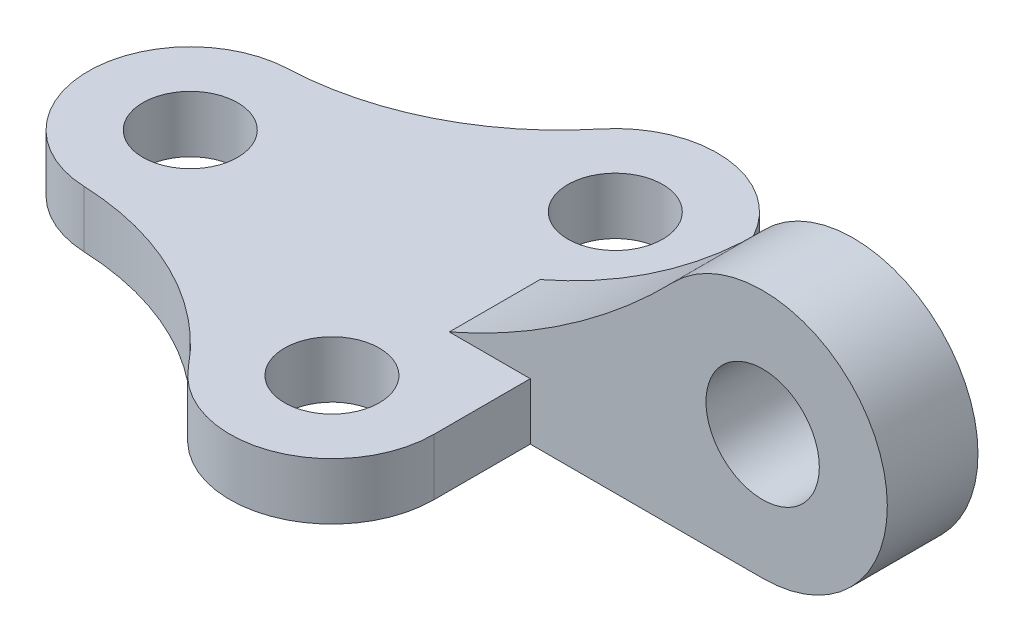
ISO-10303-21;
HEADER;
FILE_DESCRIPTION(('STEP AP214'),'2;1');
FILE_NAME('part.step','',(''),(''),'','','');
FILE_SCHEMA(('AUTOMOTIVE_DESIGN { 1 0 10303 214 1 1 1 1 }'));
ENDSEC;
DATA;
#1=APPLICATION_CONTEXT('core data for automotive mechanical design processes');
#2=APPLICATION_PROTOCOL_DEFINITION('international standard','automotive_design',2000,#1);
#3=PRODUCT_CONTEXT('',#1,'mechanical');
#4=PRODUCT('Part','Part','',(#3));
#5=PRODUCT_RELATED_PRODUCT_CATEGORY('part','',(#4));
#6=PRODUCT_DEFINITION_FORMATION('','',#4);
#7=PRODUCT_DEFINITION_CONTEXT('part definition',#1,'design');
#8=PRODUCT_DEFINITION('design','',#6,#7);
#9=PRODUCT_DEFINITION_SHAPE('','',#8);
#10=(LENGTH_UNIT() NAMED_UNIT(*) SI_UNIT(.MILLI.,.METRE.));
#11=(NAMED_UNIT(*) PLANE_ANGLE_UNIT() SI_UNIT($,.RADIAN.));
#12=(NAMED_UNIT(*) SI_UNIT($,.STERADIAN.) SOLID_ANGLE_UNIT());
#13=UNCERTAINTY_MEASURE_WITH_UNIT(LENGTH_MEASURE(1.E-05),#10,'distance_accuracy_value','');
#14=(GEOMETRIC_REPRESENTATION_CONTEXT(3) GLOBAL_UNCERTAINTY_ASSIGNED_CONTEXT((#13)) GLOBAL_UNIT_ASSIGNED_CONTEXT((#10,
#11,#12)) REPRESENTATION_CONTEXT('',''));
#15=CARTESIAN_POINT('',(0.,0.,0.));
#16=DIRECTION('',(0.,0.,1.));
#17=DIRECTION('',(1.,0.,0.));
#18=AXIS2_PLACEMENT_3D('',#15,#16,#17);
#19=CARTESIAN_POINT('',(68.,10.,-25.));
#20=DIRECTION('',(-1.,0.,0.));
#21=DIRECTION('',(0.,0.,1.));
#22=AXIS2_PLACEMENT_3D('',#19,#20,#21);
#23=PLANE('',#22);
#24=DIRECTION('',(0.,-1.,0.));
#25=VECTOR('',#24,1.);
#26=CARTESIAN_POINT('',(68.,10.,-8.));
#27=LINE('',#26,#25);
#28=CARTESIAN_POINT('',(68.,10.,-8.));
#29=VERTEX_POINT('',#28);
#30=CARTESIAN_POINT('',(68.,0.,-8.));
#31=VERTEX_POINT('',#30);
#32=EDGE_CURVE('E152',#29,#31,#27,.T.);
#33=ORIENTED_EDGE('',*,*,#32,.T.);
#34=DIRECTION('',(0.,0.,-1.));
#35=VECTOR('',#34,1.);
#36=CARTESIAN_POINT('',(68.,0.,-25.));
#37=LINE('',#36,#35);
#38=CARTESIAN_POINT('',(68.,0.,-25.));
#39=VERTEX_POINT('',#38);
#40=EDGE_CURVE('E207',#31,#39,#37,.T.);
#41=ORIENTED_EDGE('',*,*,#40,.T.);
#42=DIRECTION('',(0.,-1.,0.));
#43=VECTOR('',#42,1.);
#44=CARTESIAN_POINT('',(68.,10.,-25.));
#45=LINE('',#44,#43);
#46=CARTESIAN_POINT('',(68.,10.,-25.));
#47=VERTEX_POINT('',#46);
#48=EDGE_CURVE('E214',#47,#39,#45,.T.);
#49=ORIENTED_EDGE('',*,*,#48,.F.);
#50=DIRECTION('',(0.,0.,-1.));
#51=VECTOR('',#50,1.);
#52=CARTESIAN_POINT('',(68.,10.,-25.));
#53=LINE('',#52,#51);
#54=EDGE_CURVE('E194',#29,#47,#53,.T.);
#55=ORIENTED_EDGE('',*,*,#54,.F.);
#56=EDGE_LOOP('',(#33,#41,#49,#55));
#57=FACE_BOUND('',#56,.T.);
#58=ADVANCED_FACE('F39',(#57),#23,.F.);
#59=CARTESIAN_POINT('',(-2.72273435287364,10.,-67.9454687057473));
#60=DIRECTION('',(0.,1.,0.));
#61=DIRECTION('',(0.,0.,1.));
#62=AXIS2_PLACEMENT_3D('',#59,#60,#61);
#63=PLANE('',#62);
#64=DIRECTION('',(1.,0.,0.));
#65=VECTOR('',#64,1.);
#66=CARTESIAN_POINT('',(68.,10.,8.));
#67=LINE('',#66,#65);
#68=CARTESIAN_POINT('',(53.7099999999999,9.99999999999999,8.));
#69=VERTEX_POINT('',#68);
#70=CARTESIAN_POINT('',(68.,10.,8.));
#71=VERTEX_POINT('',#70);
#72=EDGE_CURVE('E56',#69,#71,#67,.T.);
#73=ORIENTED_EDGE('',*,*,#72,.F.);
#74=DIRECTION('',(0.,0.,-1.));
#75=VECTOR('',#74,1.);
#76=CARTESIAN_POINT('',(53.71,10.,8.));
#77=LINE('',#76,#75);
#78=CARTESIAN_POINT('',(53.7099999999999,9.99999999999999,-8.));
#79=VERTEX_POINT('',#78);
#80=EDGE_CURVE('E53',#69,#79,#77,.T.);
#81=ORIENTED_EDGE('',*,*,#80,.T.);
#82=DIRECTION('',(1.,0.,0.));
#83=VECTOR('',#82,1.);
#84=CARTESIAN_POINT('',(68.,10.,-8.));
#85=LINE('',#84,#83);
#86=EDGE_CURVE('E162',#79,#29,#85,.T.);
#87=ORIENTED_EDGE('',*,*,#86,.T.);
#88=ORIENTED_EDGE('',*,*,#54,.T.);
#89=CARTESIAN_POINT('',(50.,10.,-25.));
#90=DIRECTION('',(0.,1.,0.));
#91=DIRECTION('',(0.,0.,1.));
#92=AXIS2_PLACEMENT_3D('',#89,#90,#91);
#93=CIRCLE('',#92,18.);
#94=CARTESIAN_POINT('',(36.0439820830629,10.,-36.3679181868155));
#95=VERTEX_POINT('',#94);
#96=EDGE_CURVE('E196',#47,#95,#93,.T.);
#97=ORIENTED_EDGE('',*,*,#96,.T.);
#98=CARTESIAN_POINT('',(-2.72273435287364,10.,-67.9454687057473));
#99=DIRECTION('',(0.,-1.,0.));
#100=DIRECTION('',(0.,0.,1.));
#101=AXIS2_PLACEMENT_3D('',#98,#99,#100);
#102=CIRCLE('',#101,50.);
#103=CARTESIAN_POINT('',(-0.720723799290072,10.,-17.985565245639));
#104=VERTEX_POINT('',#103);
#105=EDGE_CURVE('E183',#95,#104,#102,.T.);
#106=ORIENTED_EDGE('',*,*,#105,.T.);
#107=CARTESIAN_POINT('',(0.,10.,0.));
#108=DIRECTION('',(0.,1.,0.));
#109=DIRECTION('',(0.,0.,1.));
#110=AXIS2_PLACEMENT_3D('',#107,#108,#109);
#111=CIRCLE('',#110,18.);
#112=CARTESIAN_POINT('',(-0.72072379929008,10.,17.985565245639));
#113=VERTEX_POINT('',#112);
#114=EDGE_CURVE('E189',#104,#113,#111,.T.);
#115=ORIENTED_EDGE('',*,*,#114,.T.);
#116=CARTESIAN_POINT('',(-2.72273435287364,10.,67.9454687057473));
#117=DIRECTION('',(0.,-1.,0.));
#118=DIRECTION('',(0.,0.,-1.));
#119=AXIS2_PLACEMENT_3D('',#116,#117,#118);
#120=CIRCLE('',#119,50.);
#121=CARTESIAN_POINT('',(36.0439820830629,10.,36.3679181868155));
#122=VERTEX_POINT('',#121);
#123=EDGE_CURVE('E193',#113,#122,#120,.T.);
#124=ORIENTED_EDGE('',*,*,#123,.T.);
#125=CARTESIAN_POINT('',(50.,10.,25.));
#126=DIRECTION('',(0.,1.,0.));
#127=DIRECTION('',(0.,0.,-1.));
#128=AXIS2_PLACEMENT_3D('',#125,#126,#127);
#129=CIRCLE('',#128,18.);
#130=CARTESIAN_POINT('',(68.,10.,25.));
#131=VERTEX_POINT('',#130);
#132=EDGE_CURVE('E191',#122,#131,#129,.T.);
#133=ORIENTED_EDGE('',*,*,#132,.T.);
#134=EDGE_CURVE('E198',#131,#71,#53,.T.);
#135=ORIENTED_EDGE('',*,*,#134,.T.);
#136=EDGE_LOOP('',(#73,#81,#87,#88,#97,#106,#115,#124,#133,#135));
#137=FACE_BOUND('',#136,.T.);
#138=CARTESIAN_POINT('',(50.,10.,-25.));
#139=DIRECTION('',(0.,1.,0.));
#140=DIRECTION('',(0.,0.,1.));
#141=AXIS2_PLACEMENT_3D('',#138,#139,#140);
#142=CIRCLE('',#141,8.36394501256826);
#143=CARTESIAN_POINT('',(50.,10.,-16.6360549874317));
#144=VERTEX_POINT('',#143);
#145=EDGE_CURVE('E174',#144,#144,#142,.T.);
#146=ORIENTED_EDGE('',*,*,#145,.F.);
#147=EDGE_LOOP('',(#146));
#148=FACE_BOUND('',#147,.T.);
#149=CARTESIAN_POINT('',(0.,10.,0.));
#150=DIRECTION('',(0.,1.,0.));
#151=DIRECTION('',(0.,0.,1.));
#152=AXIS2_PLACEMENT_3D('',#149,#150,#151);
#153=CIRCLE('',#152,8.36394501256826);
#154=CARTESIAN_POINT('',(0.,10.,8.36394501256826));
#155=VERTEX_POINT('',#154);
#156=EDGE_CURVE('E177',#155,#155,#153,.T.);
#157=ORIENTED_EDGE('',*,*,#156,.F.);
#158=EDGE_LOOP('',(#157));
#159=FACE_BOUND('',#158,.T.);
#160=CARTESIAN_POINT('',(50.,10.,25.));
#161=DIRECTION('',(0.,1.,0.));
#162=DIRECTION('',(0.,0.,-1.));
#163=AXIS2_PLACEMENT_3D('',#160,#161,#162);
#164=CIRCLE('',#163,8.36394501256826);
#165=CARTESIAN_POINT('',(50.,10.,16.6360549874317));
#166=VERTEX_POINT('',#165);
#167=EDGE_CURVE('E170',#166,#166,#164,.T.);
#168=ORIENTED_EDGE('',*,*,#167,.F.);
#169=EDGE_LOOP('',(#168));
#170=FACE_BOUND('',#169,.T.);
#171=ADVANCED_FACE('F239',(#137,#148,#159,#170),#63,.T.);
#172=CARTESIAN_POINT('',(-2.72273435287364,0.,-67.9454687057473));
#173=DIRECTION('',(0.,1.,0.));
#174=DIRECTION('',(0.,0.,1.));
#175=AXIS2_PLACEMENT_3D('',#172,#173,#174);
#176=PLANE('',#175);
#177=CARTESIAN_POINT('',(-2.72273435287364,0.,-67.9454687057473));
#178=DIRECTION('',(0.,-1.,0.));
#179=DIRECTION('',(0.,0.,1.));
#180=AXIS2_PLACEMENT_3D('',#177,#178,#179);
#181=CIRCLE('',#180,50.);
#182=CARTESIAN_POINT('',(36.0439820830629,0.,-36.3679181868155));
#183=VERTEX_POINT('',#182);
#184=CARTESIAN_POINT('',(-0.720723799290072,0.,-17.985565245639));
#185=VERTEX_POINT('',#184);
#186=EDGE_CURVE('E185',#183,#185,#181,.T.);
#187=ORIENTED_EDGE('',*,*,#186,.F.);
#188=CARTESIAN_POINT('',(50.,0.,-25.));
#189=DIRECTION('',(0.,1.,0.));
#190=DIRECTION('',(0.,0.,1.));
#191=AXIS2_PLACEMENT_3D('',#188,#189,#190);
#192=CIRCLE('',#191,18.);
#193=EDGE_CURVE('E186',#39,#183,#192,.T.);
#194=ORIENTED_EDGE('',*,*,#193,.F.);
#195=ORIENTED_EDGE('',*,*,#40,.F.);
#196=DIRECTION('',(1.,0.,0.));
#197=VECTOR('',#196,1.);
#198=CARTESIAN_POINT('',(68.,0.,-8.));
#199=LINE('',#198,#197);
#200=CARTESIAN_POINT('',(109.,0.,-8.));
#201=VERTEX_POINT('',#200);
#202=EDGE_CURVE('E137',#31,#201,#199,.T.);
#203=ORIENTED_EDGE('',*,*,#202,.T.);
#204=DIRECTION('',(0.,0.,-1.));
#205=VECTOR('',#204,1.);
#206=CARTESIAN_POINT('',(109.,0.,8.));
#207=LINE('',#206,#205);
#208=CARTESIAN_POINT('',(109.,0.,8.));
#209=VERTEX_POINT('',#208);
#210=EDGE_CURVE('E131',#209,#201,#207,.T.);
#211=ORIENTED_EDGE('',*,*,#210,.F.);
#212=DIRECTION('',(1.,0.,0.));
#213=VECTOR('',#212,1.);
#214=CARTESIAN_POINT('',(68.,0.,8.));
#215=LINE('',#214,#213);
#216=CARTESIAN_POINT('',(68.,0.,8.));
#217=VERTEX_POINT('',#216);
#218=EDGE_CURVE('E125',#217,#209,#215,.T.);
#219=ORIENTED_EDGE('',*,*,#218,.F.);
#220=CARTESIAN_POINT('',(68.,0.,25.));
#221=VERTEX_POINT('',#220);
#222=EDGE_CURVE('E209',#221,#217,#37,.T.);
#223=ORIENTED_EDGE('',*,*,#222,.F.);
#224=CARTESIAN_POINT('',(50.,0.,25.));
#225=DIRECTION('',(0.,1.,0.));
#226=DIRECTION('',(0.,0.,-1.));
#227=AXIS2_PLACEMENT_3D('',#224,#225,#226);
#228=CIRCLE('',#227,18.);
#229=CARTESIAN_POINT('',(36.0439820830629,0.,36.3679181868155));
#230=VERTEX_POINT('',#229);
#231=EDGE_CURVE('E210',#230,#221,#228,.T.);
#232=ORIENTED_EDGE('',*,*,#231,.F.);
#233=CARTESIAN_POINT('',(-2.72273435287364,0.,67.9454687057473));
#234=DIRECTION('',(0.,-1.,0.));
#235=DIRECTION('',(0.,0.,-1.));
#236=AXIS2_PLACEMENT_3D('',#233,#234,#235);
#237=CIRCLE('',#236,50.);
#238=CARTESIAN_POINT('',(-0.72072379929008,0.,17.985565245639));
#239=VERTEX_POINT('',#238);
#240=EDGE_CURVE('E202',#239,#230,#237,.T.);
#241=ORIENTED_EDGE('',*,*,#240,.F.);
#242=CARTESIAN_POINT('',(0.,0.,0.));
#243=DIRECTION('',(0.,1.,0.));
#244=DIRECTION('',(0.,0.,1.));
#245=AXIS2_PLACEMENT_3D('',#242,#243,#244);
#246=CIRCLE('',#245,18.);
#247=EDGE_CURVE('E201',#185,#239,#246,.T.);
#248=ORIENTED_EDGE('',*,*,#247,.F.);
#249=EDGE_LOOP('',(#187,#194,#195,#203,#211,#219,#223,#232,#241,#248));
#250=FACE_BOUND('',#249,.T.);
#251=CARTESIAN_POINT('',(0.,0.,0.));
#252=DIRECTION('',(0.,1.,0.));
#253=DIRECTION('',(0.,0.,1.));
#254=AXIS2_PLACEMENT_3D('',#251,#252,#253);
#255=CIRCLE('',#254,8.36394501256826);
#256=CARTESIAN_POINT('',(0.,0.,8.36394501256826));
#257=VERTEX_POINT('',#256);
#258=EDGE_CURVE('E178',#257,#257,#255,.T.);
#259=ORIENTED_EDGE('',*,*,#258,.T.);
#260=EDGE_LOOP('',(#259));
#261=FACE_BOUND('',#260,.T.);
#262=CARTESIAN_POINT('',(50.,0.,-25.));
#263=DIRECTION('',(0.,1.,0.));
#264=DIRECTION('',(0.,0.,1.));
#265=AXIS2_PLACEMENT_3D('',#262,#263,#264);
#266=CIRCLE('',#265,8.36394501256826);
#267=CARTESIAN_POINT('',(50.,0.,-16.6360549874317));
#268=VERTEX_POINT('',#267);
#269=EDGE_CURVE('E168',#268,#268,#266,.T.);
#270=ORIENTED_EDGE('',*,*,#269,.T.);
#271=EDGE_LOOP('',(#270));
#272=FACE_BOUND('',#271,.T.);
#273=CARTESIAN_POINT('',(50.,0.,25.));
#274=DIRECTION('',(0.,1.,0.));
#275=DIRECTION('',(0.,0.,-1.));
#276=AXIS2_PLACEMENT_3D('',#273,#274,#275);
#277=CIRCLE('',#276,8.36394501256826);
#278=CARTESIAN_POINT('',(50.,0.,16.6360549874317));
#279=VERTEX_POINT('',#278);
#280=EDGE_CURVE('E142',#279,#279,#277,.T.);
#281=ORIENTED_EDGE('',*,*,#280,.T.);
#282=EDGE_LOOP('',(#281));
#283=FACE_BOUND('',#282,.T.);
#284=ADVANCED_FACE('F138',(#250,#261,#272,#283),#176,.F.);
#285=CARTESIAN_POINT('',(-2.72273435287364,10.,-67.9454687057473));
#286=DIRECTION('',(0.,-1.,0.));
#287=DIRECTION('',(0.,0.,-1.));
#288=AXIS2_PLACEMENT_3D('',#285,#286,#287);
#289=CYLINDRICAL_SURFACE('',#288,50.);
#290=ORIENTED_EDGE('',*,*,#186,.T.);
#291=DIRECTION('',(0.,-1.,0.));
#292=VECTOR('',#291,1.);
#293=CARTESIAN_POINT('',(-0.720723799290072,10.,-17.985565245639));
#294=LINE('',#293,#292);
#295=EDGE_CURVE('E11',#104,#185,#294,.T.);
#296=ORIENTED_EDGE('',*,*,#295,.F.);
#297=ORIENTED_EDGE('',*,*,#105,.F.);
#298=DIRECTION('',(0.,-1.,0.));
#299=VECTOR('',#298,1.);
#300=CARTESIAN_POINT('',(36.0439820830629,10.,-36.3679181868155));
#301=LINE('',#300,#299);
#302=EDGE_CURVE('E199',#95,#183,#301,.T.);
#303=ORIENTED_EDGE('',*,*,#302,.T.);
#304=EDGE_LOOP('',(#290,#296,#297,#303));
#305=FACE_BOUND('',#304,.T.);
#306=ADVANCED_FACE('F41',(#305),#289,.F.);
#307=CARTESIAN_POINT('',(0.,10.,0.));
#308=DIRECTION('',(0.,-1.,0.));
#309=DIRECTION('',(0.,0.,-1.));
#310=AXIS2_PLACEMENT_3D('',#307,#308,#309);
#311=CYLINDRICAL_SURFACE('',#310,18.);
#312=ORIENTED_EDGE('',*,*,#247,.T.);
#313=DIRECTION('',(0.,-1.,0.));
#314=VECTOR('',#313,1.);
#315=CARTESIAN_POINT('',(-0.72072379929008,10.,17.985565245639));
#316=LINE('',#315,#314);
#317=EDGE_CURVE('E50',#113,#239,#316,.T.);
#318=ORIENTED_EDGE('',*,*,#317,.F.);
#319=ORIENTED_EDGE('',*,*,#114,.F.);
#320=ORIENTED_EDGE('',*,*,#295,.T.);
#321=EDGE_LOOP('',(#312,#318,#319,#320));
#322=FACE_BOUND('',#321,.T.);
#323=ADVANCED_FACE('F257',(#322),#311,.T.);
#324=CARTESIAN_POINT('',(-2.72273435287364,10.,67.9454687057473));
#325=DIRECTION('',(0.,-1.,0.));
#326=DIRECTION('',(0.,0.,-1.));
#327=AXIS2_PLACEMENT_3D('',#324,#325,#326);
#328=CYLINDRICAL_SURFACE('',#327,50.);
#329=ORIENTED_EDGE('',*,*,#240,.T.);
#330=DIRECTION('',(0.,-1.,0.));
#331=VECTOR('',#330,1.);
#332=CARTESIAN_POINT('',(36.0439820830629,10.,36.3679181868155));
#333=LINE('',#332,#331);
#334=EDGE_CURVE('E222',#122,#230,#333,.T.);
#335=ORIENTED_EDGE('',*,*,#334,.F.);
#336=ORIENTED_EDGE('',*,*,#123,.F.);
#337=ORIENTED_EDGE('',*,*,#317,.T.);
#338=EDGE_LOOP('',(#329,#335,#336,#337));
#339=FACE_BOUND('',#338,.T.);
#340=ADVANCED_FACE('F229',(#339),#328,.F.);
#341=CARTESIAN_POINT('',(50.,10.,25.));
#342=DIRECTION('',(0.,-1.,0.));
#343=DIRECTION('',(0.,0.,-1.));
#344=AXIS2_PLACEMENT_3D('',#341,#342,#343);
#345=CYLINDRICAL_SURFACE('',#344,18.);
#346=ORIENTED_EDGE('',*,*,#231,.T.);
#347=DIRECTION('',(0.,-1.,0.));
#348=VECTOR('',#347,1.);
#349=CARTESIAN_POINT('',(68.,10.,25.));
#350=LINE('',#349,#348);
#351=EDGE_CURVE('E217',#131,#221,#350,.T.);
#352=ORIENTED_EDGE('',*,*,#351,.F.);
#353=ORIENTED_EDGE('',*,*,#132,.F.);
#354=ORIENTED_EDGE('',*,*,#334,.T.);
#355=EDGE_LOOP('',(#346,#352,#353,#354));
#356=FACE_BOUND('',#355,.T.);
#357=ADVANCED_FACE('F232',(#356),#345,.T.);
#358=ORIENTED_EDGE('',*,*,#222,.T.);
#359=DIRECTION('',(0.,-1.,0.));
#360=VECTOR('',#359,1.);
#361=CARTESIAN_POINT('',(68.,10.,8.));
#362=LINE('',#361,#360);
#363=EDGE_CURVE('E129',#71,#217,#362,.T.);
#364=ORIENTED_EDGE('',*,*,#363,.F.);
#365=ORIENTED_EDGE('',*,*,#134,.F.);
#366=ORIENTED_EDGE('',*,*,#351,.T.);
#367=EDGE_LOOP('',(#358,#364,#365,#366));
#368=FACE_BOUND('',#367,.T.);
#369=ADVANCED_FACE('F236',(#368),#23,.F.);
#370=CARTESIAN_POINT('',(50.,10.,-25.));
#371=DIRECTION('',(0.,-1.,0.));
#372=DIRECTION('',(0.,0.,-1.));
#373=AXIS2_PLACEMENT_3D('',#370,#371,#372);
#374=CYLINDRICAL_SURFACE('',#373,18.);
#375=ORIENTED_EDGE('',*,*,#193,.T.);
#376=ORIENTED_EDGE('',*,*,#302,.F.);
#377=ORIENTED_EDGE('',*,*,#96,.F.);
#378=ORIENTED_EDGE('',*,*,#48,.T.);
#379=EDGE_LOOP('',(#375,#376,#377,#378));
#380=FACE_BOUND('',#379,.T.);
#381=ADVANCED_FACE('F258',(#380),#374,.T.);
#382=CARTESIAN_POINT('',(0.,10.,0.));
#383=DIRECTION('',(0.,-1.,0.));
#384=DIRECTION('',(0.,0.,-1.));
#385=AXIS2_PLACEMENT_3D('',#382,#383,#384);
#386=CYLINDRICAL_SURFACE('',#385,8.36394501256826);
#387=ORIENTED_EDGE('',*,*,#156,.T.);
#388=EDGE_LOOP('',(#387));
#389=FACE_BOUND('',#388,.T.);
#390=ORIENTED_EDGE('',*,*,#258,.F.);
#391=EDGE_LOOP('',(#390));
#392=FACE_BOUND('',#391,.T.);
#393=ADVANCED_FACE('F285',(#389,#392),#386,.F.);
#394=CARTESIAN_POINT('',(50.,10.,-25.));
#395=DIRECTION('',(0.,-1.,0.));
#396=DIRECTION('',(0.,0.,-1.));
#397=AXIS2_PLACEMENT_3D('',#394,#395,#396);
#398=CYLINDRICAL_SURFACE('',#397,8.36394501256826);
#399=ORIENTED_EDGE('',*,*,#145,.T.);
#400=EDGE_LOOP('',(#399));
#401=FACE_BOUND('',#400,.T.);
#402=ORIENTED_EDGE('',*,*,#269,.F.);
#403=EDGE_LOOP('',(#402));
#404=FACE_BOUND('',#403,.T.);
#405=ADVANCED_FACE('F298',(#401,#404),#398,.F.);
#406=CARTESIAN_POINT('',(50.,10.,25.));
#407=DIRECTION('',(0.,-1.,0.));
#408=DIRECTION('',(0.,0.,-1.));
#409=AXIS2_PLACEMENT_3D('',#406,#407,#408);
#410=CYLINDRICAL_SURFACE('',#409,8.36394501256826);
#411=ORIENTED_EDGE('',*,*,#167,.T.);
#412=EDGE_LOOP('',(#411));
#413=FACE_BOUND('',#412,.T.);
#414=ORIENTED_EDGE('',*,*,#280,.F.);
#415=EDGE_LOOP('',(#414));
#416=FACE_BOUND('',#415,.T.);
#417=ADVANCED_FACE('F306',(#413,#416),#410,.F.);
#418=CARTESIAN_POINT('',(109.,22.,8.));
#419=DIRECTION('',(0.,0.,1.));
#420=DIRECTION('',(1.,0.,0.));
#421=AXIS2_PLACEMENT_3D('',#418,#419,#420);
#422=PLANE('',#421);
#423=ORIENTED_EDGE('',*,*,#363,.T.);
#424=ORIENTED_EDGE('',*,*,#218,.T.);
#425=CARTESIAN_POINT('',(109.,22.,8.));
#426=DIRECTION('',(0.,0.,1.));
#427=DIRECTION('',(1.,0.,0.));
#428=AXIS2_PLACEMENT_3D('',#425,#426,#427);
#429=CIRCLE('',#428,22.);
#430=CARTESIAN_POINT('',(93.2379101954663,37.347850826543,8.));
#431=VERTEX_POINT('',#430);
#432=EDGE_CURVE('E130',#209,#431,#429,.T.);
#433=ORIENTED_EDGE('',*,*,#432,.T.);
#434=CARTESIAN_POINT('',(3.68058176061609,124.551548704628,8.));
#435=DIRECTION('',(0.,0.,-1.));
#436=DIRECTION('',(1.,0.,0.));
#437=AXIS2_PLACEMENT_3D('',#434,#435,#436);
#438=CIRCLE('',#437,125.);
#439=EDGE_CURVE('E146',#431,#69,#438,.T.);
#440=ORIENTED_EDGE('',*,*,#439,.T.);
#441=ORIENTED_EDGE('',*,*,#72,.T.);
#442=EDGE_LOOP('',(#423,#424,#433,#440,#441));
#443=FACE_BOUND('',#442,.T.);
#444=CARTESIAN_POINT('',(109.,22.,8.));
#445=DIRECTION('',(0.,0.,1.));
#446=DIRECTION('',(1.,0.,0.));
#447=AXIS2_PLACEMENT_3D('',#444,#445,#446);
#448=CIRCLE('',#447,9.99999999999999);
#449=CARTESIAN_POINT('',(119.,22.,8.));
#450=VERTEX_POINT('',#449);
#451=EDGE_CURVE('E160',#450,#450,#448,.T.);
#452=ORIENTED_EDGE('',*,*,#451,.F.);
#453=EDGE_LOOP('',(#452));
#454=FACE_BOUND('',#453,.T.);
#455=ADVANCED_FACE('F122',(#443,#454),#422,.T.);
#456=CARTESIAN_POINT('',(109.,22.,-8.));
#457=DIRECTION('',(0.,0.,1.));
#458=DIRECTION('',(1.,0.,0.));
#459=AXIS2_PLACEMENT_3D('',#456,#457,#458);
#460=PLANE('',#459);
#461=ORIENTED_EDGE('',*,*,#32,.F.);
#462=ORIENTED_EDGE('',*,*,#86,.F.);
#463=CARTESIAN_POINT('',(3.68058176061609,124.551548704628,-8.));
#464=DIRECTION('',(0.,0.,-1.));
#465=DIRECTION('',(1.,0.,0.));
#466=AXIS2_PLACEMENT_3D('',#463,#464,#465);
#467=CIRCLE('',#466,125.);
#468=CARTESIAN_POINT('',(93.2379101954663,37.347850826543,-8.));
#469=VERTEX_POINT('',#468);
#470=EDGE_CURVE('E161',#469,#79,#467,.T.);
#471=ORIENTED_EDGE('',*,*,#470,.F.);
#472=CARTESIAN_POINT('',(109.,22.,-8.));
#473=DIRECTION('',(0.,0.,1.));
#474=DIRECTION('',(1.,0.,0.));
#475=AXIS2_PLACEMENT_3D('',#472,#473,#474);
#476=CIRCLE('',#475,22.);
#477=EDGE_CURVE('E157',#201,#469,#476,.T.);
#478=ORIENTED_EDGE('',*,*,#477,.F.);
#479=ORIENTED_EDGE('',*,*,#202,.F.);
#480=EDGE_LOOP('',(#461,#462,#471,#478,#479));
#481=FACE_BOUND('',#480,.T.);
#482=CARTESIAN_POINT('',(109.,22.,-8.));
#483=DIRECTION('',(0.,0.,1.));
#484=DIRECTION('',(1.,0.,0.));
#485=AXIS2_PLACEMENT_3D('',#482,#483,#484);
#486=CIRCLE('',#485,9.99999999999999);
#487=CARTESIAN_POINT('',(119.,22.,-8.));
#488=VERTEX_POINT('',#487);
#489=EDGE_CURVE('E382',#488,#488,#486,.T.);
#490=ORIENTED_EDGE('',*,*,#489,.T.);
#491=EDGE_LOOP('',(#490));
#492=FACE_BOUND('',#491,.T.);
#493=ADVANCED_FACE('F250',(#481,#492),#460,.F.);
#494=CARTESIAN_POINT('',(109.,22.,8.));
#495=DIRECTION('',(0.,0.,-1.));
#496=DIRECTION('',(-1.,0.,0.));
#497=AXIS2_PLACEMENT_3D('',#494,#495,#496);
#498=CYLINDRICAL_SURFACE('',#497,22.);
#499=ORIENTED_EDGE('',*,*,#477,.T.);
#500=DIRECTION('',(0.,0.,-1.));
#501=VECTOR('',#500,1.);
#502=CARTESIAN_POINT('',(93.2379101954663,37.347850826543,8.));
#503=LINE('',#502,#501);
#504=EDGE_CURVE('E141',#431,#469,#503,.T.);
#505=ORIENTED_EDGE('',*,*,#504,.F.);
#506=ORIENTED_EDGE('',*,*,#432,.F.);
#507=ORIENTED_EDGE('',*,*,#210,.T.);
#508=EDGE_LOOP('',(#499,#505,#506,#507));
#509=FACE_BOUND('',#508,.T.);
#510=ADVANCED_FACE('F144',(#509),#498,.T.);
#511=CARTESIAN_POINT('',(3.68058176061609,124.551548704628,8.));
#512=DIRECTION('',(0.,0.,-1.));
#513=DIRECTION('',(-1.,0.,0.));
#514=AXIS2_PLACEMENT_3D('',#511,#512,#513);
#515=CYLINDRICAL_SURFACE('',#514,125.);
#516=ORIENTED_EDGE('',*,*,#470,.T.);
#517=ORIENTED_EDGE('',*,*,#80,.F.);
#518=ORIENTED_EDGE('',*,*,#439,.F.);
#519=ORIENTED_EDGE('',*,*,#504,.T.);
#520=EDGE_LOOP('',(#516,#517,#518,#519));
#521=FACE_BOUND('',#520,.T.);
#522=ADVANCED_FACE('F245',(#521),#515,.F.);
#523=CARTESIAN_POINT('',(109.,22.,8.));
#524=DIRECTION('',(0.,0.,-1.));
#525=DIRECTION('',(-1.,0.,0.));
#526=AXIS2_PLACEMENT_3D('',#523,#524,#525);
#527=CYLINDRICAL_SURFACE('',#526,9.99999999999999);
#528=ORIENTED_EDGE('',*,*,#451,.T.);
#529=EDGE_LOOP('',(#528));
#530=FACE_BOUND('',#529,.T.);
#531=ORIENTED_EDGE('',*,*,#489,.F.);
#532=EDGE_LOOP('',(#531));
#533=FACE_BOUND('',#532,.T.);
#534=ADVANCED_FACE('F368',(#530,#533),#527,.F.);
#535=CLOSED_SHELL('',(#58,#171,#284,#306,#323,#340,#357,#369,#381,#393,#405,#417,#455,#493,#510,
#522,#534));
#536=MANIFOLD_SOLID_BREP('B2',#535);
#537=ADVANCED_BREP_SHAPE_REPRESENTATION('',(#18,#536),#14);
#538=SHAPE_DEFINITION_REPRESENTATION(#9,#537);
ENDSEC;
END-ISO-10303-21;
